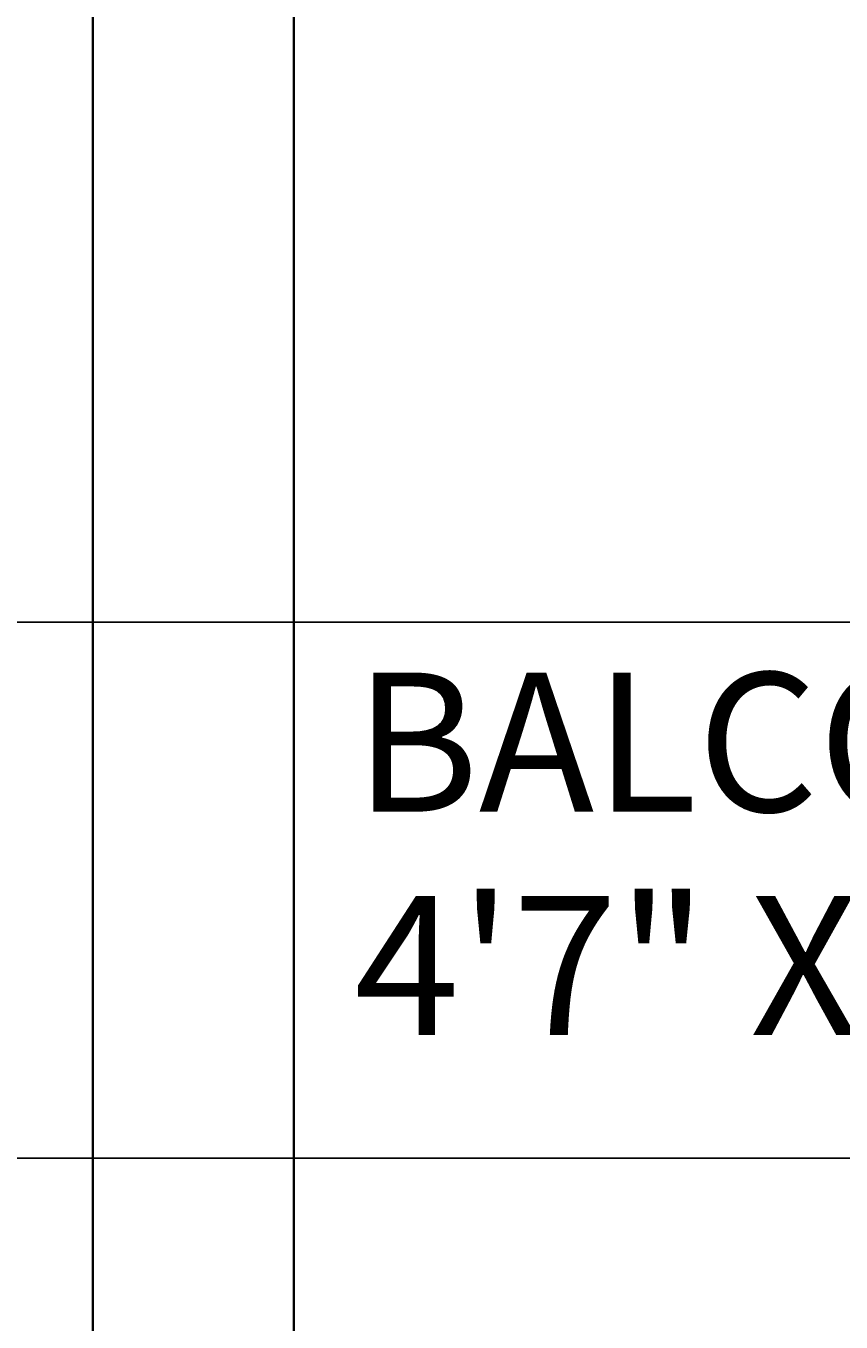
# Model space of a CAD drawing. Units: inches. Extents: x -61 to 1599, y -1316 to 257.
# Tile 57 of 204: x 12 to 48, y -282 to -224. Entities that reach past the tile are written whole.
import ezdxf

# ---------------------------------------------------------------- set-up
doc = ezdxf.new("R2010")
doc.units = ezdxf.units.IN
doc.header["$MEASUREMENT"] = 0
for name, color, linetype, lineweight in [('A-ANNO-DIMS', 2, 'Continuous', 18), ('A-AREA-IDEN', 1, 'Continuous', 18), ('WALLS', 4, 'Continuous', 35)]:
    doc.layers.add(name, color=color, linetype=linetype, lineweight=lineweight)
doc.styles.get("Standard").update_dxf_attribs({"font": 'arial.ttf'})
doc.dimstyles.get("Standard").update_dxf_attribs({"dimtxt": 0.18, "dimasz": 0.18, "dimexe": 0.18, "dimexo": 0.0625, "dimgap": 0.09, "dimtad": 0, "dimtih": 1, "dimtoh": 1, "dimdec": 0, "dimzin": 0, "dimdsep": 46, "dimlunit": 3, "dimtxsty": 'Standard', "dimcen": 0.09, "dimadec": 0, "dimazin": 0, "dimtfac": 1, "dimtdec": 0, "dimtofl": 0, "dimtmove": 0, "dimatfit": 3, "dimfxl": 1, "dimtolj": 1, "dimtzin": 0, "dimarcsym": 0})

# ---------------------------------------------------------------- blocks, each defined once
blk = doc.blocks.new('*D687')
at = {"layer": 'A-ANNO-DIMS', "color": 0, "lineweight": -2, "transparency": 16777216}
for p, q in [((289.418, 181.677), (-61.077, 181.677)), ((-60.897, 181.497), (-60.897, -528.952)), ((-60.897, -1239.765), (-60.897, -529.316)), ((319.64, -1239.945), (-61.077, -1239.945))]:
    blk.add_line(p, q, dxfattribs=at)
at = {"layer": 'A-ANNO-DIMS', "color": 0, "transparency": 16777216}
for points in [[(-60.927, 181.497), (-60.867, 181.497), (-60.897, 181.677)], [(-60.927, -1239.765), (-60.867, -1239.765), (-60.897, -1239.945)]]:
    blk.add_solid(points, dxfattribs=at)
at = {"layer": 'DEFPOINTS', "color": 0, "transparency": 16777216}
for p in [(289.481, 181.677), (-60.897, -1239.945), (319.703, -1239.945)]:
    blk.add_point(p, dxfattribs=at)
at = {"layer": 'A-ANNO-DIMS', "color": 0, "transparency": 16777216, "insert": (-60.897, -529.134), "char_height": 0.18, "attachment_point": 5}
blk.add_mtext('\\A1;1421.6', dxfattribs=at)
blk = doc.blocks.new('*D691')
at = {"layer": 'A-ANNO-DIMS', "color": 0, "lineweight": -2, "transparency": 16777216}
for p, q in [((14.64, 157.677), (-61.077, 157.677)), ((-60.897, 157.497), (-60.897, -141.641)), ((-60.897, -441.143), (-60.897, -142.005)), ((14.64, -441.323), (-61.077, -441.323))]:
    blk.add_line(p, q, dxfattribs=at)
at = {"layer": 'A-ANNO-DIMS', "color": 0, "transparency": 16777216}
for points in [[(-60.927, 157.497), (-60.867, 157.497), (-60.897, 157.677)], [(-60.927, -441.143), (-60.867, -441.143), (-60.897, -441.323)]]:
    blk.add_solid(points, dxfattribs=at)
at = {"layer": 'DEFPOINTS', "color": 0, "transparency": 16777216}
for p in [(-60.897, 157.677), (14.703, 157.677), (14.703, -441.323)]:
    blk.add_point(p, dxfattribs=at)
at = {"layer": 'A-ANNO-DIMS', "color": 0, "transparency": 16777216, "insert": (-60.897, -141.823), "char_height": 0.18, "attachment_point": 5}
blk.add_mtext('\\A1;599', dxfattribs=at)
blk = doc.blocks.new('*D699')
at = {"layer": 'A-ANNO-DIMS', "color": 0, "lineweight": -2, "transparency": 16777216}
for p, q in [((835.64, -167.169), (-61.077, -167.169)), ((-60.897, -167.349), (-60.897, -306.726)), ((-60.897, -446.466), (-60.897, -307.09)), ((841.64, -446.646), (-61.077, -446.646))]:
    blk.add_line(p, q, dxfattribs=at)
at = {"layer": 'A-ANNO-DIMS', "color": 0, "transparency": 16777216}
for points in [[(-60.927, -167.349), (-60.867, -167.349), (-60.897, -167.169)], [(-60.927, -446.466), (-60.867, -446.466), (-60.897, -446.646)]]:
    blk.add_solid(points, dxfattribs=at)
at = {"layer": 'DEFPOINTS', "color": 0, "transparency": 16777216}
for p in [(835.703, -167.169), (-60.897, -446.646), (841.703, -446.646)]:
    blk.add_point(p, dxfattribs=at)
at = {"layer": 'A-ANNO-DIMS', "color": 0, "transparency": 16777216, "insert": (-60.897, -306.908), "char_height": 0.18, "attachment_point": 5}
blk.add_mtext('\\A1;279.5', dxfattribs=at)
blk = doc.blocks.new('*D700')
at = {"layer": 'A-ANNO-DIMS', "color": 0, "lineweight": -2, "transparency": 16777216}
for p, q in [((14.703, -616.882), (14.703, 257.457)), ((14.883, 257.277), (96.772, 257.277)), ((179.572, 257.277), (97.683, 257.277)), ((179.752, -616.882), (179.752, 257.457))]:
    blk.add_line(p, q, dxfattribs=at)
at = {"layer": 'A-ANNO-DIMS', "color": 0, "transparency": 16777216}
for points in [[(14.883, 257.307), (14.883, 257.247), (14.703, 257.277)], [(179.572, 257.307), (179.572, 257.247), (179.752, 257.277)]]:
    blk.add_solid(points, dxfattribs=at)
at = {"layer": 'DEFPOINTS', "color": 0, "transparency": 16777216}
for p in [(179.752, 257.277), (14.703, -616.945), (179.752, -616.945)]:
    blk.add_point(p, dxfattribs=at)
at = {"layer": 'A-ANNO-DIMS', "color": 0, "transparency": 16777216, "insert": (97.227, 257.277), "char_height": 0.18, "attachment_point": 5}
blk.add_mtext('\\A1;165.05', dxfattribs=at)
blk = doc.blocks.new('*D706')
at = {"layer": 'A-ANNO-DIMS', "color": 0, "lineweight": -2, "transparency": 16777216}
for p, q in [((78.64, -175.323), (-61.077, -175.323)), ((-60.897, -175.503), (-60.897, -212.976)), ((-60.897, -250.814), (-60.897, -213.34)), ((78.64, -250.994), (-61.077, -250.994))]:
    blk.add_line(p, q, dxfattribs=at)
at = {"layer": 'A-ANNO-DIMS', "color": 0, "transparency": 16777216}
for points in [[(-60.927, -175.503), (-60.867, -175.503), (-60.897, -175.323)], [(-60.927, -250.814), (-60.867, -250.814), (-60.897, -250.994)]]:
    blk.add_solid(points, dxfattribs=at)
at = {"layer": 'DEFPOINTS', "color": 0, "transparency": 16777216}
for p in [(-60.897, -175.323), (78.703, -175.323), (78.703, -250.994)]:
    blk.add_point(p, dxfattribs=at)
at = {"layer": 'A-ANNO-DIMS', "color": 0, "transparency": 16777216, "insert": (-60.897, -213.158), "char_height": 0.18, "attachment_point": 5}
blk.add_mtext('\\A1;75.67', dxfattribs=at)
blk = doc.blocks.new('*D707')
at = {"layer": 'A-ANNO-DIMS', "color": 0, "lineweight": -2, "transparency": 16777216}
for p, q in [((78.64, -274.994), (-61.077, -274.994)), ((-60.897, -275.174), (-60.897, -308.474)), ((-60.897, -342.139), (-60.897, -308.838)), ((78.64, -342.319), (-61.077, -342.319))]:
    blk.add_line(p, q, dxfattribs=at)
at = {"layer": 'A-ANNO-DIMS', "color": 0, "transparency": 16777216}
for points in [[(-60.927, -275.174), (-60.867, -275.174), (-60.897, -274.994)], [(-60.927, -342.139), (-60.867, -342.139), (-60.897, -342.319)]]:
    blk.add_solid(points, dxfattribs=at)
at = {"layer": 'DEFPOINTS', "color": 0, "transparency": 16777216}
for p in [(78.703, -274.994), (-60.897, -342.319), (78.703, -342.319)]:
    blk.add_point(p, dxfattribs=at)
at = {"layer": 'A-ANNO-DIMS', "color": 0, "transparency": 16777216, "insert": (-60.897, -308.656), "char_height": 0.18, "attachment_point": 5}
blk.add_mtext('\\A1;67.33', dxfattribs=at)

msp = doc.modelspace()

# ---------------------------------------------------------------- linework, layer by layer
at = {"layer": 'WALLS'}
for p, q in [((14.7028, 157.6771), (14.7028, -441.3229)), ((23.7028, -175.3229), (23.7028, -432.3229))]:
    msp.add_line(p, q, dxfattribs=at)

# ---------------------------------------------------------------- texts
at = {"layer": 'A-AREA-IDEN'}
for s, height, p in [('BALCONY', 6.22364, (26.4051, -259.4795)), ('4\'7" X 23\'0"', 6.223643, (26.4051, -269.4772))]:
    msp.add_text(s, height=height, dxfattribs=at).set_placement(p)

# ---------------------------------------------------------------- dimensions: what is measured, and where the dimension line sits
at = {"layer": 'A-ANNO-DIMS'}
dim = msp.add_linear_dim(base=(179.7521, 257.2771), p1=(14.7028, -616.9446), p2=(179.7521, -616.9446), dimstyle='Standard', override={"dimdec": 2, "dimlfac": 1, "dimrnd": 0, "dimzin": 0, "dimdsep": 46, "dimlunit": 2}, dxfattribs=at)
dim.commit()
dim.dimension.update_dxf_attribs({"geometry": '*D700', "text_midpoint": (97.2274, 257.2771)})
for base, p1, p2, override, picture, middle in [((-60.8972, -1239.9446), (289.4807, 181.6771), (319.7028, -1239.9446), {"dimdec": 1, "dimlfac": 1, "dimrnd": 0, "dimzin": 0, "dimdsep": 46, "dimlunit": 2}, '*D687', (-60.8972, -529.1337)), ((-60.8972, 157.6771), (14.7028, -441.3229), (14.7028, 157.6771), {"dimdec": 0, "dimlfac": 1, "dimrnd": 0, "dimzin": 0, "dimdsep": 46, "dimlunit": 2}, '*D691', (-60.8972, -141.8229)), ((-60.8972, -446.6462), (835.7028, -167.169), (841.7028, -446.6462), {"dimdec": 1, "dimlfac": 1, "dimrnd": 0, "dimzin": 0, "dimdsep": 46, "dimlunit": 2}, '*D699', (-60.8972, -306.9076)), ((-60.8972, -175.3229), (78.7028, -250.9938), (78.7028, -175.3229), {"dimdec": 2, "dimlfac": 1, "dimrnd": 0, "dimzin": 0, "dimdsep": 46, "dimlunit": 2}, '*D706', (-60.8972, -213.1583)), ((-60.8972, -342.3189), (78.7028, -274.9938), (78.7028, -342.3189), {"dimdec": 2, "dimlfac": 1, "dimrnd": 0, "dimzin": 0, "dimdsep": 46, "dimlunit": 2}, '*D707', (-60.8972, -308.6563))]:
    dim = msp.add_linear_dim(base=base, p1=p1, p2=p2, angle=90, dimstyle='Standard', override=override, dxfattribs=at)
    dim.commit()
    dim.dimension.update_dxf_attribs({"geometry": picture, "text_midpoint": middle})

doc.saveas('drawing.dxf')
